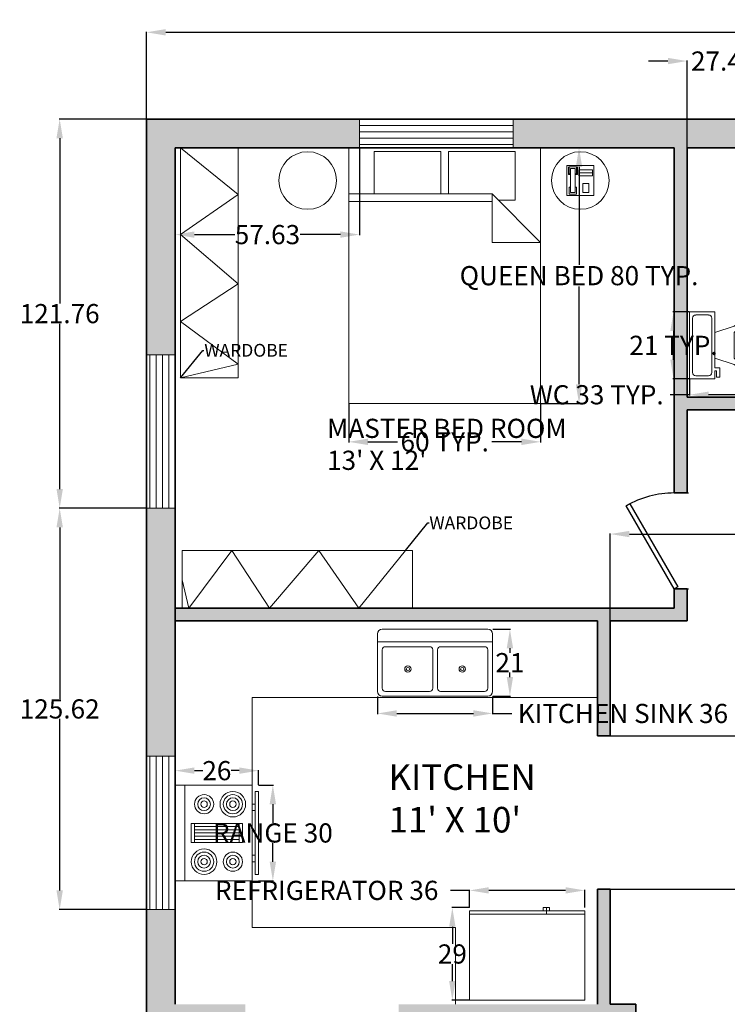
# Model space of a CAD drawing. Units: inches. Extents: x -16 to 578, y -553 to 49.
# Tile 3 of 5: x -16 to 205, y -259 to 49. Entities that reach past the tile are written whole.
import ezdxf
from ezdxf import colors
from ezdxf.entities.mleader import LeaderData, LeaderLine
from ezdxf.math import Vec2, Vec3

# ---------------------------------------------------------------- set-up
doc = ezdxf.new("R2010")
doc.units = ezdxf.units.IN
doc.header["$MEASUREMENT"] = 0
for name, color, linetype, lineweight in [('A-ANNO-DIMS', 2, 'Continuous', 18), ('A-ANNO-TEXT', 7, 'Continuous', 18), ('A-AREA-IDEN', 7, 'Continuous', 25), ('A-DOOR', 3, 'Continuous', 25), ('A-EQPM', 8, 'Continuous', 18), ('A-FLOR-CASE', 8, 'Continuous', 18), ('A-FLOR-FIXT', 9, 'Continuous', 18), ('A-FURN', 8, 'Continuous', 18), ('A-GLAZ', 4, 'Continuous', 18), ('A-WALL', 7, 'Continuous', 35)]:
    doc.layers.add(name, color=color, linetype=linetype, lineweight=lineweight)
doc.layers.add('A-WALL-PATT', color=251, linetype='Continuous', lineweight=13, true_color=0x636466)
doc.styles.get("Standard").update_dxf_attribs({"font": 'arial.ttf'})
doc.dimstyles.get("Standard").update_dxf_attribs({"dimtxt": 6, "dimasz": 6, "dimexe": 0.18, "dimexo": 0.0625, "dimgap": 0.09, "dimtad": 0, "dimtih": 1, "dimtoh": 1, "dimdec": 0, "dimzin": 0, "dimdsep": 46, "dimlunit": 4, "dimtxsty": 'Standard', "dimcen": 0.09, "dimadec": 0, "dimazin": 0, "dimtfac": 1, "dimtdec": 0, "dimtofl": 0, "dimtmove": 0, "dimatfit": 3, "dimfxl": 1, "dimtolj": 1, "dimtzin": 0, "dimarcsym": 0})

# ---------------------------------------------------------------- blocks, each defined once
blk = doc.blocks.new('*U3')
for p, q in [((-40, 0), (-40, 6)), ((0, 0), (0, 6))]:
    blk.add_line(p, q)
blk.add_lwpolyline([(0, 0), (-34.64, -20), (-35.52, -18.48), (-0.88, 1.52)], close=True)
blk.add_arc((0, 0), 40, 180, 210)
blk = doc.blocks.new('Range-Oven - 30 in top')
for p, q in [((0, -3), (30, -3)), ((12, -6), (18, -6)), ((13, -20), (13, -6)), ((14, -6), (14, -20)), ((15, -20), (15, -6)), ((16, -6), (16, -20)), ((17, -20), (17, -6)), ((18, -20), (12, -20)), ((6, -24), (6, -25)), ((8, -25), (8, -24)), ((22, -25), (22, -24)), ((24, -24), (24, -25))]:
    blk.add_line(p, q)
for points in [[(0, -24), (0, 0), (30, 0), (30, -24)], [(12, -21), (12, -5), (18, -5), (18, -21)], [(2, -26), (2, -25), (28, -25), (28, -26)]]:
    blk.add_lwpolyline(points, close=True)
for centre, radius in [((6, -9), 4), ((6, -9), 3), ((24, -9), 3), ((6, -9), 2), ((6, -9), 1), ((24, -9), 2), ((24, -9), 1), ((6, -18), 3), ((24, -18), 4), ((24, -18), 3), ((6, -18), 2), ((6, -18), 1), ((24, -18), 2), ((24, -18), 1)]:
    blk.add_circle(centre, radius)
blk = doc.blocks.new('Sink-double - 36 in top')
for p, q in [((-18, -4), (18, -4)), ((-0.75, -18.5), (-0.75, -6.5)), ((0.75, -6.5), (0.75, -18.5))]:
    blk.add_line(p, q)
for points in [[(-16.5, 0), (16.5, 0)], [(-18, -19.5), (-18, -1.5)], [(18, -1.5), (18, -19.5)], [(-15.5, -5.5), (-1.75, -5.5)], [(1.75, -5.5), (15.5, -5.5)], [(-16.5, -18.5), (-16.5, -6.5)], [(16.5, -6.5), (16.5, -18.5)], [(16.5, -21), (-16.5, -21)], [(-1.75, -19.5), (-15.5, -19.5)], [(15.5, -19.5), (1.75, -19.5)]]:
    blk.add_lwpolyline(points)
for centre, radius in [((-8.5, -12.5), 1), ((-8.5, -12.5), 0.5), ((8.5, -12.5), 1), ((8.5, -12.5), 0.5)]:
    blk.add_circle(centre, radius)
for centre, radius, start, end in [((-16.5, -1.5), 1.5, 90, 180), ((16.5, -1.5), 1.5, 0, 90), ((-15.5, -6.5), 1, 90, 180), ((-1.75, -6.5), 1, 0, 90), ((1.75, -6.5), 1, 90, 180), ((15.5, -6.5), 1, 0, 90), ((-16.5, -19.5), 1.5, 180, 270), ((-15.5, -18.5), 1, 180, 270), ((-1.75, -18.5), 1, 270, 0), ((1.75, -18.5), 1, 180, 270), ((15.5, -18.5), 1, 270, 0), ((16.5, -19.5), 1.5, 270, 0)]:
    blk.add_arc(centre, radius, start, end)
blk = doc.blocks.new('Refrigerator-2 door - 36 in top')
for p, q in [((0, -26.999999), (36, -26.999999)), ((12, -26.999999), (12, -28.999999)), ((11, -27.999999), (11, -28.999999)), ((11, -28.999999), (13, -28.999999)), ((13, -28.999999), (13, -27.999999))]:
    blk.add_line(p, q)
blk.add_lwpolyline([(0, -27.999999), (0, 0), (36, 0), (36, -27.999999)], close=True)
blk = doc.blocks.new('Toilet - top')
for p, q in [((9.5, -6), (9.5, -2)), ((-10, -8.5), (-8, -8.5)), ((-10, -9.5), (-10, -8.5)), ((-8, -8.5), (-8, -8)), ((-7, -8), (-7, -9.5)), ((-4, -8), (-6, -14)), ((4, -8), (6, -14)), ((-7, -9.5), (-10, -9.5)), ((4, -14), (-4, -14))]:
    blk.add_line(p, q)
for points in [[(-7, -8), (10.5, -8), (10.5, 0), (-10.5, 0), (-10.5, -8), (-8, -8)], [(-9.5, -2), (-9.5, -6)], [(8.5, -1), (-8.5, -1)], [(-8.5, -7), (8.5, -7)]]:
    blk.add_lwpolyline(points)
for centre, radius, start, end in [((-8.62, -1.88), 0.884, 81.8699, 188.1301), ((8.62, -1.88), 0.884, 351.8699, 98.1301), ((-8.62, -6.12), 0.884, 171.8699, 278.1301), ((8.62, -6.12), 0.884, 261.8699, 8.1301), ((3.52, -21.58), 12.17, 141.4691, 247.9714), ((4.2, -21.82), 11.33, 136.3677, 238.9468), ((-3.52, -21.58), 12.17, 292.0284, 38.5307), ((-4.2, -21.82), 11.33, 301.053, 43.6321), ((0, -27.88), 4, 245.7318, 294.2682), ((0, -29), 4, 254.8605, 285.1395)]:
    blk.add_arc(centre, radius, start, end)
blk = doc.blocks.new('Bed - Queen')
for p, q in [((0, -80.00003), (0, 0)), ((0, 0), (59.99999, 0)), ((59.99999, 0), (59.99999, -80.00003)), ((7.99999, -1.2), (28.79998, -1.2)), ((7.99999, -14.4), (7.99999, -1.2)), ((28.79998, -1.2), (28.79998, -14.4)), ((31.19999, -1.2), (51.99999, -1.2)), ((31.19999, -14.4), (31.19999, -1.2)), ((51.99999, -1.2), (51.99999, -16.4)), ((0, -14.4), (44.8, -14.4)), ((59.99999, -29.6), (44.8, -14.4)), ((44.8, -14.4), (44.8, -29.6)), ((44.8, -16.8), (0, -16.8)), ((51.99999, -16.4), (46.79936, -16.4)), ((44.8, -29.6), (59.99999, -29.6)), ((59.99999, -80.00003), (0, -80.00003))]:
    blk.add_line(p, q)
blk = doc.blocks.new('Phone - Desk')
for p, q in [((-4.5, -5), (-4.5, 5)), ((-4.5, 5), (4.5, 5)), ((-4, 4.5), (-4, 2)), ((-3.75, 4.5), (-3.75, 2.25)), ((-1.25, 4.5), (-3.75, 4.5)), ((-3.25, 4), (-3.25, -4)), ((-3.25, 4), (-1.75, 4)), ((-1.75, -4), (-1.75, 4)), ((-1.25, 2.25), (-1.25, 4.5)), ((-1, 2), (-1, 4.5)), ((4, 3.5), (-0.5, 3.5)), ((-0.5, 3.5), (-0.5, 1.5)), ((4, 1.5), (4, 3.5)), ((4.5, 5), (4.5, -5)), ((-4, 2), (-3.25, 2)), ((-3.75, 2.25), (-3.25, 2.25)), ((-1.75, 2.25), (-1.25, 2.25)), ((-1.75, 2), (-1, 2)), ((-0.5, 2.5), (4, 2.5)), ((-0.5, 1.5), (4, 1.5)), ((-3.75, -2.25), (-3.25, -2.25)), ((-3.75, -4.5), (-3.75, -2.25)), ((-1.75, -2.25), (-1.25, -2.25)), ((-1.25, -2.25), (-1.25, -4.5)), ((2.75, -1), (0.75, -1)), ((0.75, -1), (0.75, -4)), ((2.75, -4), (2.75, -1)), ((4.5, -5), (-4.5, -5)), ((-1.25, -4.5), (-3.75, -4.5)), ((-3.25, -4), (-1.75, -4)), ((0.75, -4), (2.75, -4))]:
    blk.add_line(p, q)
blk = doc.blocks.new('WIN-48X9')
for p, q in [((-48, -4), (0, -4)), ((-48, -6), (0, -6)), ((-48, -8), (0, -8))]:
    blk.add_line(p, q)
for points in [[(0, 0), (0, -9), (-48, -9), (-48, 0)], [(-48, -2), (0, -2)]]:
    blk.add_lwpolyline(points, close=True)
blk = doc.blocks.new('WARDROBE-72X18')
for p, q in [((0, 0), (18, -14.58)), ((18, -14.58), (0, -27.16)), ((0, -27.16), (18, -42.59)), ((18, -42.59), (0, -54.31)), ((0, -54.31), (18, -67.75)), ((18, -67.75), (0, -72))]:
    blk.add_line(p, q)
blk.add_lwpolyline([(0, 0), (18, 0), (18, -72), (0, -72)], close=True)
blk = doc.blocks.new('NIGHTSTAND-ROUND-18')
blk.add_circle((0, 0), 9)
blk = doc.blocks.new('*D32')
at = {"layer": 'A-ANNO-DIMS', "color": 0, "lineweight": -2, "transparency": 16777216}
for p, q in [((146.48, 9.23), (158.6, 9.23)), ((158.42, 3.23), (158.42, -27.39)), ((158.42, -64.77), (158.42, -34.14)), ((146.48, -70.77), (158.6, -70.77))]:
    blk.add_line(p, q, dxfattribs=at)
at = {"layer": 'A-ANNO-DIMS', "color": 0, "transparency": 16777216}
for points in [[(157.42, 3.23), (159.42, 3.23), (158.42, 9.23)], [(157.42, -64.77), (159.42, -64.77), (158.42, -70.77)]]:
    blk.add_solid(points, dxfattribs=at)
at = {"layer": 'Defpoints', "color": 0, "transparency": 16777216}
for p in [(146.42, 9.23), (158.42, 9.23), (146.42, -70.77)]:
    blk.add_point(p, dxfattribs=at)
at = {"layer": 'A-ANNO-DIMS', "color": 0, "transparency": 16777216, "insert": (158.42, -30.77), "char_height": 6, "attachment_point": 5}
blk.add_mtext('\\A1;QUEEN BED 80 TYP.', dxfattribs=at)
blk = doc.blocks.new('*D33')
at = {"layer": 'A-ANNO-DIMS', "color": 0, "lineweight": -2, "transparency": 16777216}
for p, q in [((86.42, -70.83), (86.42, -82.95)), ((146.42, -70.83), (146.42, -82.95)), ((92.42, -82.77), (101.71, -82.77)), ((140.42, -82.77), (131.13, -82.77))]:
    blk.add_line(p, q, dxfattribs=at)
at = {"layer": 'A-ANNO-DIMS', "color": 0, "transparency": 16777216}
for points in [[(92.42, -81.77), (92.42, -83.77), (86.42, -82.77)], [(140.42, -81.77), (140.42, -83.77), (146.42, -82.77)]]:
    blk.add_solid(points, dxfattribs=at)
at = {"layer": 'Defpoints', "color": 0, "transparency": 16777216}
for p in [(86.42, -70.77), (146.42, -70.77), (146.42, -82.77)]:
    blk.add_point(p, dxfattribs=at)
at = {"layer": 'A-ANNO-DIMS', "color": 0, "transparency": 16777216, "insert": (116.42, -82.77), "char_height": 6, "attachment_point": 5}
blk.add_mtext('\\A1;60 TYP.', dxfattribs=at)
blk = doc.blocks.new('*D38')
at = {"layer": 'A-ANNO-DIMS', "color": 0, "lineweight": -2, "transparency": 16777216}
for p, q in [((192.91, -63.14), (192.91, -68.22)), ((225.96, -63.14), (225.96, -68.22)), ((192.91, -68.04), (186.91, -68.04)), ((219.96, -68.04), (198.91, -68.04))]:
    blk.add_line(p, q, dxfattribs=at)
at = {"layer": 'A-ANNO-DIMS', "color": 0, "transparency": 16777216}
for points in [[(198.91, -67.04), (198.91, -69.04), (192.91, -68.04)], [(219.96, -67.04), (219.96, -69.04), (225.96, -68.04)]]:
    blk.add_solid(points, dxfattribs=at)
at = {"layer": 'Defpoints', "color": 0, "transparency": 16777216}
for p in [(192.91, -63.08), (225.96, -63.08), (192.91, -68.04)]:
    blk.add_point(p, dxfattribs=at)
at = {"layer": 'A-ANNO-DIMS', "color": 0, "transparency": 16777216, "insert": (163.95, -68.04), "char_height": 6, "attachment_point": 5}
blk.add_mtext('\\A1;WC 33 TYP.', dxfattribs=at)
blk = doc.blocks.new('*D39')
at = {"layer": 'A-ANNO-DIMS', "color": 0, "lineweight": -2, "transparency": 16777216}
for p, q in [((192.85, -42.08), (187.78, -42.08)), ((187.96, -48.08), (187.96, -49.48)), ((187.96, -57.08), (187.96, -55.68)), ((192.85, -63.08), (187.78, -63.08))]:
    blk.add_line(p, q, dxfattribs=at)
at = {"layer": 'A-ANNO-DIMS', "color": 0, "transparency": 16777216}
for points in [[(186.96, -48.08), (188.96, -48.08), (187.96, -42.08)], [(186.96, -57.08), (188.96, -57.08), (187.96, -63.08)]]:
    blk.add_solid(points, dxfattribs=at)
at = {"layer": 'Defpoints', "color": 0, "transparency": 16777216}
for p in [(187.96, -42.08), (192.91, -42.08), (192.91, -63.08)]:
    blk.add_point(p, dxfattribs=at)
at = {"layer": 'A-ANNO-DIMS', "color": 0, "transparency": 16777216, "insert": (187.96, -52.58), "char_height": 6, "attachment_point": 5}
blk.add_mtext('\\A1;21 TYP.', dxfattribs=at)
blk = doc.blocks.new('*D52')
at = {"layer": 'A-ANNO-DIMS', "color": 0, "lineweight": -2, "transparency": 16777216}
for p, q in [((58.25, -190.15), (62.87, -190.15)), ((62.69, -196.15), (62.69, -201.96)), ((62.69, -214.15), (62.69, -208.34)), ((58.25, -220.15), (62.87, -220.15))]:
    blk.add_line(p, q, dxfattribs=at)
at = {"layer": 'A-ANNO-DIMS', "color": 0, "transparency": 16777216}
for points in [[(61.69, -196.15), (63.69, -196.15), (62.69, -190.15)], [(61.69, -214.15), (63.69, -214.15), (62.69, -220.15)]]:
    blk.add_solid(points, dxfattribs=at)
at = {"layer": 'Defpoints', "color": 0, "transparency": 16777216}
for p in [(58.19, -190.15), (62.69, -190.15), (58.19, -220.15)]:
    blk.add_point(p, dxfattribs=at)
at = {"layer": 'A-ANNO-DIMS', "color": 0, "transparency": 16777216, "insert": (62.69, -205.15), "char_height": 6, "attachment_point": 5}
blk.add_mtext('\\A1;RANGE 30', dxfattribs=at)
blk = doc.blocks.new('*D53')
at = {"layer": 'A-ANNO-DIMS', "color": 0, "lineweight": -2, "transparency": 16777216}
for p, q in [((32.19, -190.09), (32.19, -185.47)), ((38.19, -185.65), (40.75, -185.65)), ((52.19, -185.65), (49.62, -185.65)), ((58.19, -190.09), (58.19, -185.47))]:
    blk.add_line(p, q, dxfattribs=at)
at = {"layer": 'A-ANNO-DIMS', "color": 0, "transparency": 16777216}
for points in [[(38.19, -184.65), (38.19, -186.65), (32.19, -185.65)], [(52.19, -184.65), (52.19, -186.65), (58.19, -185.65)]]:
    blk.add_solid(points, dxfattribs=at)
at = {"layer": 'Defpoints', "color": 0, "transparency": 16777216}
for p in [(32.19, -185.65), (32.19, -190.15), (58.19, -190.15)]:
    blk.add_point(p, dxfattribs=at)
at = {"layer": 'A-ANNO-DIMS', "color": 0, "transparency": 16777216, "insert": (45.19, -185.65), "char_height": 6, "attachment_point": 5}
blk.add_mtext('\\A1;26', dxfattribs=at)
blk = doc.blocks.new('*D54')
at = {"layer": 'A-ANNO-DIMS', "color": 0, "lineweight": -2, "transparency": 16777216}
for p, q in [((95.41, -162.43), (95.41, -167.94)), ((131.41, -162.43), (131.41, -167.94)), ((101.41, -167.76), (125.41, -167.76)), ((131.41, -167.76), (137.41, -167.76))]:
    blk.add_line(p, q, dxfattribs=at)
at = {"layer": 'A-ANNO-DIMS', "color": 0, "transparency": 16777216}
for points in [[(101.41, -166.76), (101.41, -168.76), (95.41, -167.76)], [(125.41, -166.76), (125.41, -168.76), (131.41, -167.76)]]:
    blk.add_solid(points, dxfattribs=at)
at = {"layer": 'Defpoints', "color": 0, "transparency": 16777216}
for p in [(95.41, -162.36), (131.41, -162.36), (131.41, -167.76)]:
    blk.add_point(p, dxfattribs=at)
at = {"layer": 'A-ANNO-DIMS', "color": 0, "transparency": 16777216, "insert": (172.16, -167.76), "char_height": 6, "attachment_point": 5}
blk.add_mtext('\\A1;KITCHEN SINK 36', dxfattribs=at)
blk = doc.blocks.new('*D55')
at = {"layer": 'A-ANNO-DIMS', "color": 0, "lineweight": -2, "transparency": 16777216}
for p, q in [((131.47, -141.36), (136.99, -141.36)), ((136.81, -147.36), (136.81, -148.76)), ((136.81, -156.36), (136.81, -154.97)), ((131.47, -162.36), (136.99, -162.36))]:
    blk.add_line(p, q, dxfattribs=at)
at = {"layer": 'A-ANNO-DIMS', "color": 0, "transparency": 16777216}
for points in [[(135.81, -147.36), (137.81, -147.36), (136.81, -141.36)], [(135.81, -156.36), (137.81, -156.36), (136.81, -162.36)]]:
    blk.add_solid(points, dxfattribs=at)
at = {"layer": 'Defpoints', "color": 0, "transparency": 16777216}
for p in [(131.41, -141.36), (136.81, -141.36), (131.41, -162.36)]:
    blk.add_point(p, dxfattribs=at)
at = {"layer": 'A-ANNO-DIMS', "color": 0, "transparency": 16777216, "insert": (136.81, -151.86), "char_height": 6, "attachment_point": 5}
blk.add_mtext('\\A1;21', dxfattribs=at)
blk = doc.blocks.new('*D56')
at = {"layer": 'A-ANNO-DIMS', "color": 0, "lineweight": -2, "transparency": 16777216}
for p, q in [((124.21, -223.12), (118.21, -223.12)), ((124.21, -228.46), (124.21, -222.94)), ((154.21, -223.12), (130.21, -223.12)), ((160.21, -228.46), (160.21, -222.94))]:
    blk.add_line(p, q, dxfattribs=at)
at = {"layer": 'A-ANNO-DIMS', "color": 0, "transparency": 16777216}
for points in [[(130.21, -222.12), (130.21, -224.12), (124.21, -223.12)], [(154.21, -222.12), (154.21, -224.12), (160.21, -223.12)]]:
    blk.add_solid(points, dxfattribs=at)
at = {"layer": 'Defpoints', "color": 0, "transparency": 16777216}
for p in [(124.21, -223.12), (124.21, -228.52), (160.21, -228.52)]:
    blk.add_point(p, dxfattribs=at)
at = {"layer": 'A-ANNO-DIMS', "color": 0, "transparency": 16777216, "insert": (79.52, -223.12), "char_height": 6, "attachment_point": 5}
blk.add_mtext('\\A1;REFRIGERATOR 36', dxfattribs=at)
blk = doc.blocks.new('*D57')
at = {"layer": 'A-ANNO-DIMS', "color": 0, "lineweight": -2, "transparency": 16777216}
for p, q in [((124.15, -228.52), (118.63, -228.52)), ((118.81, -234.52), (118.81, -239.87)), ((118.81, -251.52), (118.81, -246.17)), ((124.15, -257.52), (118.63, -257.52))]:
    blk.add_line(p, q, dxfattribs=at)
at = {"layer": 'A-ANNO-DIMS', "color": 0, "transparency": 16777216}
for points in [[(117.81, -234.52), (119.81, -234.52), (118.81, -228.52)], [(117.81, -251.52), (119.81, -251.52), (118.81, -257.52)]]:
    blk.add_solid(points, dxfattribs=at)
at = {"layer": 'Defpoints', "color": 0, "transparency": 16777216}
for p in [(124.21, -228.52), (118.81, -257.52), (124.21, -257.52)]:
    blk.add_point(p, dxfattribs=at)
at = {"layer": 'A-ANNO-DIMS', "color": 0, "transparency": 16777216, "insert": (118.81, -243.02), "char_height": 6, "attachment_point": 5}
blk.add_mtext('\\A1;29', dxfattribs=at)
blk = doc.blocks.new('*D62')
at = {"layer": 'A-ANNO-DIMS', "color": 0, "lineweight": -2, "transparency": 16777216}
for p, q in [((23.19, 18.3), (23.19, 45.56)), ((29.19, 45.38), (256.36, 45.38)), ((497.19, 45.38), (270.02, 45.38)), ((503.19, 18.3), (503.19, 45.56))]:
    blk.add_line(p, q, dxfattribs=at)
at = {"layer": 'A-ANNO-DIMS', "color": 0, "transparency": 16777216}
for points in [[(29.19, 46.38), (29.19, 44.38), (23.19, 45.38)], [(497.19, 46.38), (497.19, 44.38), (503.19, 45.38)]]:
    blk.add_solid(points, dxfattribs=at)
at = {"layer": 'Defpoints', "color": 0, "transparency": 16777216}
for p in [(503.19, 45.38), (23.19, 18.23), (503.19, 18.23)]:
    blk.add_point(p, dxfattribs=at)
at = {"layer": 'A-ANNO-DIMS', "color": 0, "transparency": 16777216, "insert": (263.19, 45.38), "char_height": 6, "attachment_point": 5}
blk.add_mtext('\\A1;480', dxfattribs=at)
blk = doc.blocks.new('*D69')
at = {"layer": 'A-ANNO-DIMS', "color": 0, "lineweight": -2, "transparency": 16777216}
for p, q in [((168.25, -174.77), (530.52, -174.77)), ((530.34, -180.77), (530.34, -195.61)), ((530.34, -216.77), (530.34, -201.92)), ((168.25, -222.77), (530.52, -222.77))]:
    blk.add_line(p, q, dxfattribs=at)
at = {"layer": 'A-ANNO-DIMS', "color": 0, "transparency": 16777216}
for points in [[(529.34, -180.77), (531.34, -180.77), (530.34, -174.77)], [(529.34, -216.77), (531.34, -216.77), (530.34, -222.77)]]:
    blk.add_solid(points, dxfattribs=at)
at = {"layer": 'Defpoints', "color": 0, "transparency": 16777216}
for p in [(168.19, -174.77), (168.19, -222.77), (530.34, -222.77)]:
    blk.add_point(p, dxfattribs=at)
at = {"layer": 'A-ANNO-DIMS', "color": 0, "transparency": 16777216, "insert": (530.34, -198.77), "char_height": 6, "attachment_point": 5}
blk.add_mtext('\\A1;48', dxfattribs=at)
blk = doc.blocks.new('*D71')
at = {"layer": 'A-ANNO-DIMS', "color": 0, "lineweight": -2, "transparency": 16777216}
for p, q in [((32.19, 9.17), (32.19, -18.1)), ((89.82, 9.17), (89.82, -18.1)), ((38.19, -17.92), (50.79, -17.92)), ((83.82, -17.92), (71.22, -17.92))]:
    blk.add_line(p, q, dxfattribs=at)
at = {"layer": 'A-ANNO-DIMS', "color": 0, "transparency": 16777216}
for points in [[(38.19, -16.92), (38.19, -18.92), (32.19, -17.92)], [(83.82, -16.92), (83.82, -18.92), (89.82, -17.92)]]:
    blk.add_solid(points, dxfattribs=at)
at = {"layer": 'Defpoints', "color": 0, "transparency": 16777216}
for p in [(32.19, 9.23), (89.82, 9.23), (32.19, -17.92)]:
    blk.add_point(p, dxfattribs=at)
at = {"layer": 'A-ANNO-DIMS', "color": 0, "transparency": 16777216, "insert": (61, -17.92), "char_height": 6, "attachment_point": 5}
blk.add_mtext('\\A1;57.63', dxfattribs=at)
blk = doc.blocks.new('*D72')
at = {"layer": 'A-ANNO-DIMS', "color": 0, "lineweight": -2, "transparency": 16777216}
for p, q in [((186.19, 36.38), (180.19, 36.38)), ((192.19, 9.3), (192.19, 36.56)), ((219.64, 9.3), (219.64, 36.56)), ((225.64, 36.38), (231.64, 36.38))]:
    blk.add_line(p, q, dxfattribs=at)
at = {"layer": 'A-ANNO-DIMS', "color": 0, "transparency": 16777216}
for points in [[(186.19, 37.38), (186.19, 35.38), (192.19, 36.38)], [(225.64, 37.38), (225.64, 35.38), (219.64, 36.38)]]:
    blk.add_solid(points, dxfattribs=at)
at = {"layer": 'Defpoints', "color": 0, "transparency": 16777216}
for p in [(219.64, 36.38), (192.19, 9.23), (219.64, 9.23)]:
    blk.add_point(p, dxfattribs=at)
at = {"layer": 'A-ANNO-DIMS', "color": 0, "transparency": 16777216, "insert": (205.91, 36.38), "char_height": 6, "attachment_point": 5}
blk.add_mtext('\\A1;27.453', dxfattribs=at)
blk = doc.blocks.new('*D78')
at = {"layer": 'A-ANNO-DIMS', "color": 0, "lineweight": -2, "transparency": 16777216}
for p, q in [((23.13, 18.23), (-4.14, 18.23)), ((-3.96, 12.23), (-3.96, -39.49)), ((-3.96, -97.53), (-3.96, -45.8)), ((23.13, -103.53), (-4.14, -103.53))]:
    blk.add_line(p, q, dxfattribs=at)
at = {"layer": 'A-ANNO-DIMS', "color": 0, "transparency": 16777216}
for points in [[(-4.96, 12.23), (-2.96, 12.23), (-3.96, 18.23)], [(-4.96, -97.53), (-2.96, -97.53), (-3.96, -103.53)]]:
    blk.add_solid(points, dxfattribs=at)
at = {"layer": 'Defpoints', "color": 0, "transparency": 16777216}
for p in [(23.19, 18.23), (-3.96, -103.53), (23.19, -103.53)]:
    blk.add_point(p, dxfattribs=at)
at = {"layer": 'A-ANNO-DIMS', "color": 0, "transparency": 16777216, "insert": (-3.96, -42.65), "char_height": 6, "attachment_point": 5}
blk.add_mtext('\\A1;121.76', dxfattribs=at)
blk = doc.blocks.new('*D79')
at = {"layer": 'A-ANNO-DIMS', "color": 0, "lineweight": -2, "transparency": 16777216}
for p, q in [((23.13, -103.53), (-4.14, -103.53)), ((-3.96, -109.53), (-3.96, -163.18)), ((-3.96, -223.15), (-3.96, -169.49)), ((23.13, -229.15), (-4.14, -229.15))]:
    blk.add_line(p, q, dxfattribs=at)
at = {"layer": 'A-ANNO-DIMS', "color": 0, "transparency": 16777216}
for points in [[(-4.96, -109.53), (-2.96, -109.53), (-3.96, -103.53)], [(-4.96, -223.15), (-2.96, -223.15), (-3.96, -229.15)]]:
    blk.add_solid(points, dxfattribs=at)
at = {"layer": 'Defpoints', "color": 0, "transparency": 16777216}
for p in [(23.19, -103.53), (-3.96, -229.15), (23.19, -229.15)]:
    blk.add_point(p, dxfattribs=at)
at = {"layer": 'A-ANNO-DIMS', "color": 0, "transparency": 16777216, "insert": (-3.96, -166.34), "char_height": 6, "attachment_point": 5}
blk.add_mtext('\\A1;125.62', dxfattribs=at)
blk = doc.blocks.new('*D83')
at = {"layer": 'A-ANNO-DIMS', "color": 0, "lineweight": -2, "transparency": 16777216}
for p, q in [((168.19, -138.7), (168.19, -111.44)), ((174.19, -111.62), (256.76, -111.62)), ((352.19, -111.62), (269.61, -111.62)), ((358.19, -138.7), (358.19, -111.44))]:
    blk.add_line(p, q, dxfattribs=at)
at = {"layer": 'A-ANNO-DIMS', "color": 0, "transparency": 16777216}
for points in [[(174.19, -110.62), (174.19, -112.62), (168.19, -111.62)], [(352.19, -110.62), (352.19, -112.62), (358.19, -111.62)]]:
    blk.add_solid(points, dxfattribs=at)
at = {"layer": 'Defpoints', "color": 0, "transparency": 16777216}
for p in [(358.19, -111.62), (168.19, -138.77), (358.19, -138.77)]:
    blk.add_point(p, dxfattribs=at)
at = {"layer": 'A-ANNO-DIMS', "color": 0, "transparency": 16777216, "insert": (263.19, -111.62), "char_height": 6, "attachment_point": 5}
blk.add_mtext('\\A1;190', dxfattribs=at)

msp = doc.modelspace()

# ---------------------------------------------------------------- hatches: boundary and pattern name
at = {"layer": 'A-WALL-PATT'}
h = msp.add_hatch(color=256, dxfattribs=at)
h.dxf.hatch_style = 1
h.paths.add_polyline_path([(32.1882, 9.2337), (89.8211, 9.2337), (89.8211, 18.2337), (23.1882, 18.2337), (23.1882, -55.5259), (32.1882, -55.5259)])
h.paths.add_polyline_path([(219.6411, 18.2337), (137.8211, 18.2337), (137.8211, 9.2337), (146.4179, 9.2337), (188.1882, 9.2337), (188.1882, -98.7663), (192.1882, -98.7663), (192.1882, -72.7663), (238.1882, -72.7663), (238.1882, -68.7663), (192.1882, -68.7663), (192.1882, 9.2337), (219.6411, 9.2337)])
h.paths.add_polyline_path([(307.3924, 18.2337), (243.6411, 18.2337), (243.6411, 9.2337), (274.1882, 9.2337), (274.1882, -26.7663), (274.1882, -68.7663), (268.1882, -68.7663), (268.1882, -72.7663), (274.1882, -72.7663), (274.1882, -98.7663), (250.1882, -98.7663), (250.1882, -102.7663), (274.1882, -102.7663), (278.1882, -102.7663), (302.188, -102.8481), (302.188, -98.8481), (278.1882, -98.7663), (278.1882, -86.8559, -0.01827889), (278.1882, -85.7663), (278.1882, -72.7663), (284.1882, -72.7663), (284.1882, -68.7663), (278.1882, -68.7663), (278.1882, 9.2337), (307.3924, 9.2337)])
h.paths.add_polyline_path([(402.6701, 18.2337), (331.3924, 18.2337), (331.3924, 9.2337), (358.1882, 9.2337), (358.1882, -26.7663), (358.1882, -68.7663), (314.1882, -68.7663), (314.1882, -72.7663), (358.1882, -72.7663), (358.1882, -98.7663), (362.1882, -98.7663), (362.1882, 9.2337), (402.6701, 9.2337)])
h.paths.add_polyline_path([(503.1882, 18.2337), (450.6701, 18.2337), (450.6701, 9.2337), (462.8072, 9.2337), (494.1882, 9.2337), (494.1882, -38.053), (503.1882, -38.053)])
h.paths.add_polyline_path([(503.1882, -86.053), (494.1882, -86.053), (494.1882, -134.7663), (362.1882, -134.7663), (362.1882, -128.7663), (358.1882, -128.7663), (358.1882, -138.7663), (358.1882, -234.7663), (362.1882, -234.7663), (362.1882, -138.7663), (494.1882, -138.7663), (494.1882, -181.1501), (503.1882, -181.1501)])
h.paths.add_polyline_path([(503.1882, -229.1501), (494.1882, -229.1501), (494.1882, -270.7663), (362.1882, -270.7663), (362.1882, -264.7663), (358.1882, -264.7663), (358.1882, -294.7663), (358.1882, -323.1753), (362.1882, -323.1753), (362.1882, -298.7663), (362.1882, -294.7663), (362.1882, -274.7663), (494.1882, -274.7663), (494.1882, -294.7663), (494.1882, -298.7663), (494.1882, -310.411), (503.1882, -310.411)])
h.paths.add_polyline_path([(503.1882, -358.411), (494.1882, -358.411), (494.1882, -394.7663), (362.1882, -394.7663), (362.1882, -353.1753), (358.1882, -353.1753), (358.1882, -398.7663), (494.1882, -398.7663), (494.1882, -512.7663), (451.8049, -512.7663), (451.8049, -521.7663), (503.1882, -521.7663)])
h.paths.add_polyline_path([(403.8049, -512.7663), (176.1882, -512.7663), (176.1882, -441.7663), (172.1882, -441.7663), (172.1882, -512.7663), (150.1882, -512.7663), (150.1882, -521.7663), (403.8049, -521.7663)])
h.paths.add_polyline_path([(176.1882, -258.7663), (168.1882, -258.7663), (168.1882, -246.7663), (168.1882, -234.7663), (168.1882, -222.7663), (164.1882, -222.7663), (164.1882, -234.7663), (164.1882, -258.7663), (102.0641, -258.7663), (102.0641, -262.7663), (168.1882, -262.7663), (172.1882, -262.7663), (172.1882, -333.7663), (176.1882, -333.7663), (176.1882, -262.7663)])
h.paths.add_polyline_path([(32.1882, -262.7663), (54.0641, -262.7663), (54.0641, -258.7663), (32.1882, -258.7663), (32.1882, -229.1501), (23.1882, -229.1501), (23.1882, -283.4909), (23.1882, -470.2771), (32.1882, -470.2771), (32.1882, -283.4909)])
h.paths.add_polyline_path([(32.1882, -103.5259), (23.1882, -103.5259), (23.1882, -181.1501), (32.1882, -181.1501)])
h.paths.add_polyline_path([(192.1882, -128.7663), (188.1882, -128.7663), (188.1882, -134.7663), (32.1882, -134.7663), (32.1882, -138.7663), (164.1882, -138.7663), (164.1882, -162.7663), (164.1882, -174.7663), (168.1882, -174.7663), (168.1882, -162.7663), (168.1882, -138.7663), (192.1882, -138.7663)])

# ---------------------------------------------------------------- linework, layer by layer
at = {"layer": 'A-FLOR-CASE'}
for p, q in [((49.8766, -116.7663), (36.4416, -134.7663)), ((61.5965, -134.7663), (49.8766, -116.7663)), ((77.0324, -116.7663), (61.5965, -134.7663)), ((89.6098, -134.7663), (77.0324, -116.7663)), ((104.1882, -116.7663), (89.6098, -134.7663)), ((36.4416, -134.7663), (34.352, -125.9234)), ((56.1882, -162.7663), (164.1882, -162.7663)), ((56.1882, -234.7663), (56.1882, -162.7663)), ((56.1882, -234.7663), (119.8061, -234.7663)), ((119.8061, -234.7663), (119.8061, -258.7663))]:
    msp.add_line(p, q, dxfattribs=at)
msp.add_lwpolyline([(106.352, -116.7663), (106.352, -134.7663), (34.352, -134.7663), (34.352, -116.7663)], close=True, dxfattribs=at)
at = {"layer": 'A-WALL'}
for p, q in [((32.1882, 9.2337), (188.1882, 9.2337)), ((32.1882, -258.7663), (32.1882, 9.2337)), ((188.1882, -98.7663), (188.1882, 9.2337)), ((192.1882, 9.2337), (274.1882, 9.2337)), ((192.1882, -68.7663), (192.1882, 9.2337)), ((192.1882, -68.7663), (238.1882, -68.7663)), ((192.1882, -72.7663), (238.1882, -72.7663)), ((192.1882, -98.7663), (192.1882, -72.7663)), ((188.1882, -98.7663), (192.1882, -98.7663)), ((188.1882, -134.7663), (188.1882, -128.7663)), ((188.1882, -128.7663), (192.1882, -128.7663)), ((192.1882, -138.7663), (192.1882, -128.7663)), ((32.1882, -134.7663), (188.1882, -134.7663)), ((32.1882, -138.7663), (164.1882, -138.7663)), ((164.1882, -162.7663), (164.1882, -138.7663)), ((168.1882, -138.7663), (192.1882, -138.7663)), ((168.1882, -150.7663), (168.1882, -138.7663)), ((168.1882, -162.7663), (168.1882, -138.7663)), ((164.1882, -174.7663), (164.1882, -162.7663)), ((168.1882, -162.7663), (168.1882, -174.7663)), ((168.1882, -174.7663), (164.1882, -174.7663)), ((168.1882, -222.7663), (164.1882, -222.7663)), ((164.1882, -222.7663), (164.1882, -234.7663)), ((168.1882, -234.7663), (168.1882, -222.7663)), ((164.1882, -258.7663), (164.1882, -234.7663)), ((168.1882, -258.7663), (168.1882, -234.7663)), ((168.1882, -258.7663), (168.1882, -246.7663)), ((168.1882, -258.7663), (176.1882, -258.7663)), ((176.1882, -258.7663), (176.1882, -262.7663))]:
    msp.add_line(p, q, dxfattribs=at)
msp.add_lwpolyline([(23.1882, -283.4909), (23.1882, 18.2337), (503.1882, 18.2337), (503.1882, -521.7663), (150.1882, -521.7663)], dxfattribs=at)

# ---------------------------------------------------------------- block references
at = {"layer": 'A-DOOR', "xscale": 0.75, "yscale": 0.75, "zscale": 0.75, "rotation": 270}
msp.add_blockref('*U3', (188.1882, -128.7663), dxfattribs=at)
at = {"layer": 'A-EQPM', "xscale": 0.9424999999999881, "yscale": 0.9424999999999881, "zscale": 0.9424999999999881}
msp.add_blockref('Phone - Desk', (158.8539, -0.9972), dxfattribs=at)
at = {"layer": 'A-EQPM'}
for name, p, rotation in [('Range-Oven - 30 in top', (32.1882, -220.1501), 90), ('Refrigerator-2 door - 36 in top', (160.2133, -257.5195), 180)]:
    msp.add_blockref(name, p, dxfattribs=dict(at, rotation=rotation))
at = {"layer": 'A-FLOR-CASE'}
msp.add_blockref('WARDROBE-72X18', (33.8211, 9.2337), dxfattribs=at)
at = {"layer": 'A-FLOR-FIXT', "rotation": 90}
msp.add_blockref('Toilet - top', (192.9126, -52.58), dxfattribs=at)
at = {"layer": 'A-FLOR-FIXT'}
msp.add_blockref('Sink-double - 36 in top', (113.4071, -141.3644), dxfattribs=at)
at = {"layer": 'A-FURN'}
for name, p in [('NIGHTSTAND-ROUND-18', (73.58, -0.9972)), ('Bed - Queen', (86.4179, 9.2337)), ('NIGHTSTAND-ROUND-18', (158.8539, -0.9972))]:
    msp.add_blockref(name, p, dxfattribs=at)
at = {"layer": 'A-GLAZ'}
msp.add_blockref('WIN-48X9', (137.8211, 18.2337), dxfattribs=at)
for p, rotation in [((32.1882, -103.5259), 270), ((32.1882, -229.1501), 270.0000000000001)]:
    msp.add_blockref('WIN-48X9', p, dxfattribs=dict(at, rotation=rotation))

# ---------------------------------------------------------------- texts
at = {"layer": 'A-AREA-IDEN', "attachment_point": 1}
for s, width, insert, char_height in [("MASTER BED ROOM\\P13' X 12'", 92.635717, (79.6332, -75.5469), 6), ("KITCHEN\\P11' X 10'", 68.466466, (98.8568, -183.6678), 8)]:
    msp.add_mtext_dynamic_manual_height_columns(s, width=width, gutter_width=1, heights=[0], dxfattribs=dict(at, insert=insert, char_height=char_height))

# ---------------------------------------------------------------- dimensions: what is measured, and where the dimension line sits
at = {"layer": 'A-ANNO-DIMS'}
for base, p1, p2, picture, middle in [((503.1882, 45.3837), (23.1882, 18.2337), (503.1882, 18.2337), '*D62', (263.1882, 45.3837)), ((358.1882, -111.6163), (168.1882, -138.7663), (358.1882, -138.7663), '*D83', (263.1882, -111.6163))]:
    dim = msp.add_linear_dim(base=base, p1=p1, p2=p2, dimstyle='Standard', override={"dimdec": 0, "dimlfac": 1, "dimrnd": 0, "dimzin": 0, "dimdsep": 46, "dimlunit": 2}, dxfattribs=at)
    dim.commit()
    dim.dimension.update_dxf_attribs({"geometry": picture, "text_midpoint": middle})
for base, p1, p2, angle, override, picture, middle in [((219.6411, 36.3837), (192.1882, 9.2337), (219.6411, 9.2337), 0, {"dimdec": 3, "dimlfac": 1, "dimrnd": 0, "dimzin": 0, "dimdsep": 46, "dimlunit": 2}, '*D72', (205.9146, 36.3837)), ((-3.9618, -103.5259), (23.1882, 18.2337), (23.1882, -103.5259), 90, {"dimdec": 2, "dimlfac": 1, "dimrnd": 0, "dimzin": 0, "dimdsep": 46, "dimlunit": 2}, '*D78', (-3.9618, -42.6461)), ((32.1882, -17.9163), (89.8211, 9.2337), (32.1882, 9.2337), 180, {"dimdec": 2, "dimlfac": 1, "dimrnd": 0, "dimzin": 0, "dimdsep": 46, "dimlunit": 2}, '*D71', (61.0046, -17.9163)), ((-3.9618, -229.1501), (23.1882, -103.5259), (23.1882, -229.1501), 90, {"dimdec": 2, "dimlfac": 1, "dimrnd": 0, "dimzin": 0, "dimdsep": 46, "dimlunit": 2}, '*D79', (-3.9618, -166.338)), ((136.8071, -141.3644), (131.4071, -162.3644), (131.4071, -141.3644), 90, {"dimdec": 0, "dimlfac": 1, "dimrnd": 0, "dimzin": 0, "dimdsep": 46, "dimlunit": 2}, '*D55', (136.8071, -151.8644)), ((530.3382, -222.7663), (168.1882, -174.7663), (168.1882, -222.7663), 90, {"dimdec": 0, "dimlfac": 1, "dimrnd": 0, "dimzin": 0, "dimdsep": 46, "dimlunit": 2}, '*D69', (530.3382, -198.7663)), ((32.1882, -185.6501), (58.1882, -190.1501), (32.1882, -190.1501), 180, {"dimdec": 0, "dimlfac": 1, "dimrnd": 0, "dimzin": 0, "dimdsep": 46, "dimlunit": 2}, '*D53', (45.1882, -185.6501)), ((118.8133, -257.5195), (124.2133, -228.5195), (124.2133, -257.5195), 270, {"dimdec": 0, "dimlfac": 1, "dimrnd": 0, "dimzin": 0, "dimdsep": 46, "dimlunit": 2}, '*D57', (118.8133, -243.0195))]:
    dim = msp.add_linear_dim(base=base, p1=p1, p2=p2, angle=angle, dimstyle='Standard', override=override, dxfattribs=at)
    dim.commit()
    dim.dimension.update_dxf_attribs({"geometry": picture, "text_midpoint": middle})
for base, p1, p2, angle, text, picture, middle in [((158.4179, 9.2337), (146.4179, -70.7663), (146.4179, 9.2337), 90, 'QUEEN BED <> TYP.', '*D32', (158.4179, -30.7663)), ((187.9556, -42.08), (192.9126, -63.08), (192.9126, -42.08), 90, '<> TYP.', '*D39', (187.9556, -52.58)), ((192.9126, -68.037), (225.9588, -63.08), (192.9126, -63.08), 180, 'WC <> TYP.', '*D38', (163.9501, -68.037)), ((62.6882, -190.1501), (58.1882, -220.1501), (58.1882, -190.1501), 90, 'RANGE <>', '*D52', (62.6882, -205.1501)), ((124.2133, -223.1195), (160.2133, -228.5195), (124.2133, -228.5195), 180, 'REFRIGERATOR <>', '*D56', (79.5223, -223.1195))]:
    dim = msp.add_linear_dim(base=base, p1=p1, p2=p2, angle=angle, text=text, dimstyle='Standard', override={"dimdec": 0, "dimlfac": 1, "dimrnd": 0, "dimzin": 0, "dimdsep": 46, "dimlunit": 2}, dxfattribs=at)
    dim.commit()
    dim.dimension.update_dxf_attribs({"geometry": picture, "text_midpoint": middle})
for base, p1, p2, text, picture, middle in [((146.4179, -82.7663), (86.4179, -70.7663), (146.4179, -70.7663), '<> TYP.', '*D33', (116.4179, -82.7663)), ((131.4071, -167.7644), (95.4071, -162.3644), (131.4071, -162.3644), 'KITCHEN SINK <>', '*D54', (172.1649, -167.7644))]:
    dim = msp.add_linear_dim(base=base, p1=p1, p2=p2, text=text, dimstyle='Standard', override={"dimdec": 0, "dimlfac": 1, "dimrnd": 0, "dimzin": 0, "dimdsep": 46, "dimlunit": 2}, dxfattribs=at)
    dim.commit()
    dim.dimension.update_dxf_attribs({"geometry": picture, "text_midpoint": middle})

# ---------------------------------------------------------------- leaders
at = {"layer": 'A-ANNO-TEXT'}
ml = msp.add_multileader_mtext('Standard', dxfattribs=at)
ml.set_content('WARDOBE', color=256)
ml.set_leader_properties()
ml.build(insert=Vec2(0, 0))
ml.multileader.update_dxf_attribs({"dogleg_length": 0.36, "arrow_head_size": 0})
ctx = ml.context
ctx.base_point, ctx.arrow_head_size, ctx.landing_gap_size, ctx.plane_origin = Vec3(41.1523, -54.1589), 0, 0.09, Vec3(33.8211, -62.7663)
notes = []
notes.append((ctx, [(0, (1, 1, 0), (40.7923, -54.1589), (1, 0), 0.36, [(0, [(33.8211, -62.7663)], 0, [])])]))
ctx.mtext.insert, ctx.mtext.width, ctx.mtext.flow_direction = Vec3(41.2423, -52.1248), 4, 5
ml = msp.add_multileader_mtext('Standard', dxfattribs=at)
ml.set_content('WARDOBE', color=256)
ml.set_leader_properties()
ml.build(insert=Vec2(0, 0))
ml.multileader.update_dxf_attribs({"dogleg_length": 0.36, "arrow_head_size": 0})
ctx = ml.context
ctx.base_point, ctx.arrow_head_size, ctx.landing_gap_size, ctx.plane_origin = Vec3(111.5193, -108.1589), 0, 0.09, Vec3(104.1882, -116.7663)
notes.append((ctx, [(0, (1, 1, 0), (111.1593, -108.1589), (1, 0), 0.36, [(0, [(104.1882, -116.7663)], 0, [])])]))
ctx.mtext.insert, ctx.mtext.width, ctx.mtext.flow_direction = Vec3(111.6093, -106.1248), 4, 5
for ctx, leaders in notes:
    for number, flags, end, landing, length, lines in leaders:
        leader = LeaderData()
        leader.index, (leader.has_last_leader_line, leader.has_dogleg_vector, leader.attachment_direction) = number, flags
        leader.last_leader_point, leader.dogleg_vector, leader.dogleg_length = Vec3(end), Vec3(landing), length
        for number, points, colour, breaks in lines:
            line = LeaderLine()
            line.index, line.vertices, line.color, line.breaks = number, Vec3.list(points), colors.encode_raw_color(colour), breaks
            leader.lines.append(line)
        ctx.leaders.append(leader)

doc.saveas('drawing.dxf')
